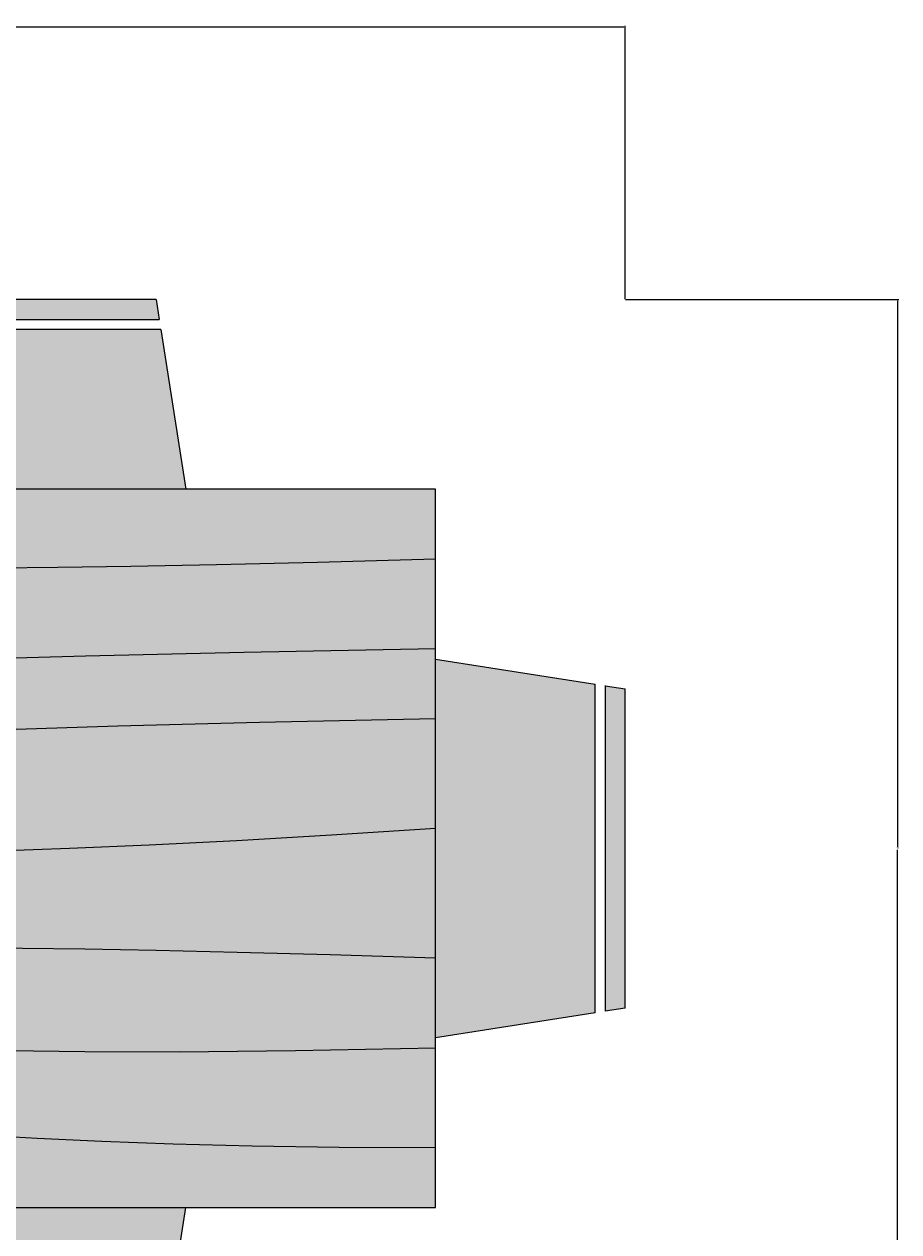
# Model space of a CAD drawing. Units: inches. Extents: x 192 to 1361, y -1362 to 367.
# Tile 18 of 23: x 662 to 781, y -337 to -173. Entities that reach past the tile are written whole.
import ezdxf

# ---------------------------------------------------------------- set-up
doc = ezdxf.new("R2010")
doc.units = ezdxf.units.IN
doc.header["$MEASUREMENT"] = 0
doc.layers.add('A-ANNO-DIMS', color=2, linetype='Continuous', lineweight=18)
doc.layers.add('furniture', color=32, linetype='Continuous', lineweight=18)
doc.layers.add('A-FURN-PATT', color=254, linetype='Continuous', lineweight=13, true_color=0xfeeab9)
doc.styles.get("Standard").update_dxf_attribs({"font": 'arial.ttf'})
doc.dimstyles.get("Standard").update_dxf_attribs({"dimtxt": 0.18, "dimasz": 0.18, "dimexe": 0.18, "dimexo": 0.0625, "dimgap": 0.09, "dimtad": 0, "dimtih": 1, "dimtoh": 1, "dimzin": 0, "dimdsep": 46, "dimlunit": 3, "dimtxsty": 'Standard', "dimcen": 0.09, "dimadec": 0, "dimazin": 0, "dimtfac": 1, "dimtofl": 0, "dimtmove": 0, "dimatfit": 3, "dimfxl": 1, "dimtolj": 1, "dimtzin": 0, "dimarcsym": 0})

# ---------------------------------------------------------------- blocks, each defined once
blk = doc.blocks.new('Dining Set - 36 x 72 in.')
for p, q in [((-22, 27.5), (-22.1562, 26.50042)), ((-22, 27.5), (-6, 27.5)), ((-5.8437, 26.49966), (-6, 27.5)), ((6, 27.5), (5.8438, 26.50042)), ((6, 27.5), (22, 27.5)), ((22.1563, 26.49966), (22, 27.5)), ((-5.8416, 26.5), (-22.1534, 26.5)), ((22.1584, 26.5), (5.8466, 26.5)), ((-22.2343, 26.00059), (-23.4847, 17.99762)), ((-22.2304, 26), (-5.7608, 26)), ((-4.5152, 17.99762), (-5.7655, 25.99926)), ((5.7657, 26.00059), (4.5153, 17.99762)), ((5.7696, 26), (22.2392, 26)), ((23.4848, 17.99762), (22.2345, 25.99926)), ((36, 18), (-36, 18)), ((-36, 18), (-36, -18)), ((36, -18), (36, 18)), ((-44.0006, 8.23428), (-35.9976, 9.48474)), ((44.0006, 8.23428), (35.9976, 9.48474)), ((-45.5, 8), (-44.5004, 8.15617)), ((-45.5, 8), (-45.5, -8)), ((-44.5, -8.15843), (-44.5, 8.15338)), ((-44, 8.23041), (-44, -8.23915)), ((44, 8.23041), (44, -8.23915)), ((44.5, -8.15843), (44.5, 8.15338)), ((45.5, 8), (44.5005, 8.15617)), ((45.5, 8), (45.5, -8)), ((-44.4997, -8.15631), (-45.5, -8)), ((-35.9976, -9.48476), (-43.9993, -8.2345)), ((35.9976, -9.48476), (43.9993, -8.2345)), ((44.4997, -8.15631), (45.5, -8)), ((-36, -18), (36, -18)), ((-22.2343, -26.0006), (-23.4847, -17.99762)), ((-4.5152, -17.99762), (-5.7655, -25.99928)), ((5.7657, -26.0006), (4.5153, -17.99762)), ((23.4848, -17.99762), (22.2345, -25.99928)), ((-22.2304, -26), (-5.7608, -26)), ((5.7696, -26), (22.2392, -26)), ((-22, -27.5), (-22.1562, -26.50044)), ((-5.8416, -26.5), (-22.1534, -26.5)), ((-5.8437, -26.49967), (-6, -27.5)), ((6, -27.5), (5.8438, -26.50044)), ((22.1584, -26.5), (5.8466, -26.5)), ((22.1563, -26.49967), (22, -27.5)), ((-22, -27.5), (-6, -27.5)), ((6, -27.5), (22, -27.5))]:
    blk.add_line(p, q)
for points in [[(-36, 15), (-31.1772, 14.97754), (-26.8079, 14.91406), (-22.8538, 14.81543), (-19.276, 14.6875), (-16.0362, 14.53613), (-13.0957, 14.36718), (-10.4159, 14.18652), (-7.9583, 14), (-5.6904, 13.81315), (-3.6035, 13.63021), (-1.6954, 13.45508), (0.0365, 13.29166), (1.5945, 13.14388), (2.9811, 13.01562), (4.1988, 12.9108), (5.25, 12.83333), (6.1393, 12.78613), (6.8802, 12.76823), (7.4883, 12.77767), (7.9792, 12.8125), (8.3685, 12.87077), (8.6719, 12.95052), (8.9049, 13.0498), (9.0833, 13.16666), (9.2205, 13.29899), (9.3216, 13.44401), (9.3895, 13.59879), (9.4271, 13.76041), (9.4373, 13.92594), (9.4232, 14.09245), (9.3875, 14.257), (9.3333, 14.41666), (9.2638, 14.56917), (9.1836, 14.71484), (9.0975, 14.85465), (9.0104, 14.98958), (8.9272, 15.1206), (8.8529, 15.2487), (8.7922, 15.37483), (8.75, 15.5), (8.7305, 15.62467), (8.7344, 15.74739), (8.7617, 15.86621), (8.8125, 15.97916), (8.8867, 16.08431), (8.9844, 16.17968), (9.1055, 16.26334), (9.25, 16.33333), (9.4189, 16.38802), (9.6172, 16.42708), (9.8506, 16.45052), (10.125, 16.45833), (10.4463, 16.45052), (10.8203, 16.42708), (11.2529, 16.38802), (11.75, 16.33333), (12.3184, 16.26318), (12.9694, 16.17838), (13.7151, 16.07991), (14.5677, 15.96875), (15.5395, 15.84586), (16.6426, 15.71224), (17.8893, 15.56884), (19.2917, 15.41666), (20.859, 15.25667), (22.5879, 15.08984), (24.4721, 14.91715), (26.5052, 14.73958), (28.6809, 14.5581), (30.9929, 14.3737), (33.4347, 14.18733), (36, 14)], [(-36, 10), (-28.9766, 10.14274), (-23.1725, 10.20442), (-18.4241, 10.19775), (-14.5677, 10.13541), (-11.4399, 10.03011), (-8.877, 9.89453), (-6.7154, 9.74137), (-4.7917, 9.58333), (-2.9698, 9.43082), (-1.2246, 9.28515), (0.4415, 9.14534), (2.026, 9.01041), (3.5266, 8.87939), (4.9408, 8.7513), (6.266, 8.62516), (7.5, 8.5), (8.6411, 8.37549), (9.6914, 8.2539), (10.6538, 8.13818), (11.5312, 8.03125), (12.3267, 7.93603), (13.043, 7.85547), (13.6831, 7.79248), (14.25, 7.75), (14.7471, 7.7303), (15.1797, 7.73307), (15.5537, 7.75732), (15.875, 7.80208), (16.1494, 7.86637), (16.3828, 7.94922), (16.5811, 8.04964), (16.75, 8.16666), (16.8944, 8.29915), (17.0143, 8.44531), (17.1089, 8.60319), (17.1771, 8.77083), (17.218, 8.94629), (17.2305, 9.1276), (17.2137, 9.31282), (17.1667, 9.5), (17.0895, 9.6875), (16.987, 9.875), (16.8649, 10.0625), (16.7292, 10.25), (16.5856, 10.4375), (16.4401, 10.625), (16.2985, 10.8125), (16.1667, 11), (16.05, 11.18733), (15.9518, 11.3737), (15.8752, 11.5581), (15.8229, 11.73958), (15.798, 11.91715), (15.8034, 12.08984), (15.842, 12.25667), (15.9167, 12.41666), (16.0295, 12.56836), (16.1784, 12.70833), (16.3605, 12.83268), (16.5729, 12.9375), (16.8127, 13.01888), (17.0768, 13.07291), (17.3625, 13.0957), (17.6667, 13.08333), (17.9894, 13.03312), (18.3418, 12.94726), (18.7382, 12.82918), (19.1927, 12.68229), (19.7195, 12.51001), (20.3327, 12.31575), (21.0465, 12.10294), (21.875, 11.875), (22.8357, 11.63354), (23.959, 11.37304), (25.2786, 11.08618), (26.8282, 10.76562), (28.6414, 10.40405), (30.752, 9.99414), (33.1936, 9.52856), (36, 9)], [(-36, 5.5), (-30.7157, 5.3348), (-26.069, 5.20963), (-21.9946, 5.11767), (-18.4271, 5.05208), (-15.3009, 5.00602), (-12.5508, 4.97265), (-10.1112, 4.94515), (-7.9167, 4.91666), (-5.909, 4.88167), (-4.0586, 4.83984), (-2.3429, 4.79215), (-0.7396, 4.73958), (0.7739, 4.6831), (2.22, 4.6237), (3.6213, 4.56233), (5, 4.5), (6.373, 4.43782), (7.7344, 4.3776), (9.0723, 4.32129), (10.375, 4.27083), (11.6309, 4.22819), (12.8281, 4.19531), (13.9551, 4.17415), (15, 4.16666), (15.954, 4.17448), (16.819, 4.19791), (17.6001, 4.23698), (18.3021, 4.29166), (18.9299, 4.36198), (19.4883, 4.44791), (19.9823, 4.54948), (20.4167, 4.66666), (20.7969, 4.79899), (21.1302, 4.94401), (21.4245, 5.09879), (21.6875, 5.26041), (21.9271, 5.42594), (22.1511, 5.59245), (22.3672, 5.757), (22.5834, 5.91666), (22.8065, 6.06868), (23.0404, 6.21093), (23.2879, 6.34147), (23.5521, 6.45833), (23.8358, 6.55957), (24.142, 6.64323), (24.4735, 6.70735), (24.8334, 6.75), (25.2235, 6.76969), (25.642, 6.76692), (26.0858, 6.74267), (26.5521, 6.69791), (27.0379, 6.63362), (27.5404, 6.55078), (28.0565, 6.45036), (28.5834, 6.33333), (29.1242, 6.19987), (29.7071, 6.04687), (30.3661, 5.87044), (31.1354, 5.66666), (32.0493, 5.43164), (33.142, 5.16146), (34.4475, 4.85221), (36, 4.5)], [(-36, -1), (-30.7915, -0.6591), (-26.0195, -0.38216), (-21.6519, -0.16284), (-17.6563, 0.00521), (-14.0005, 0.12833), (-10.6523, 0.21289), (-7.5796, 0.26522), (-4.75, 0.29166), (-2.134, 0.29793), (0.2878, 0.28711), (2.5317, 0.26163), (4.6146, 0.22396), (6.5529, 0.17651), (8.3633, 0.12174), (10.0623, 0.06209), (11.6667, 0), (13.1899, -0.06201), (14.6341, -0.1211), (15.9982, -0.17432), (17.2813, -0.21875), (18.4823, -0.25147), (19.6003, -0.26953), (20.6343, -0.27002), (21.5834, -0.25), (22.4481, -0.20768), (23.2357, -0.14584), (23.9549, -0.06836), (24.6146, 0.02083), (25.2235, 0.11784), (25.7904, 0.21875), (26.3241, 0.31966), (26.8334, 0.41666), (27.3265, 0.50618), (27.8099, 0.58593), (28.2894, 0.65397), (28.7709, 0.70833), (29.2601, 0.74707), (29.763, 0.76823), (30.2855, 0.76985), (30.8334, 0.75), (31.4088, 0.70784), (31.9994, 0.64713), (32.589, 0.57275), (33.1615, 0.48958), (33.7008, 0.4025), (34.1908, 0.3164), (34.6153, 0.23616), (34.9584, 0.16666), (35.2099, 0.11165), (35.3848, 0.07031), (35.504, 0.04069), (35.5886, 0.02083), (35.6594, 0.00879), (35.7377, 0.0026), (35.8442, 0.00032), (36, 0)], [(-36, -6.5), (-27.1843, -6.31267), (-20.084, -6.1263), (-14.469, -5.9419), (-10.1094, -5.76042), (-6.7752, -5.58285), (-4.2363, -5.41016), (-2.2629, -5.24333), (-0.625, -5.08334), (0.8708, -4.93099), (2.2715, -4.78646), (3.5872, -4.64974), (4.8281, -4.52084), (6.0046, -4.39974), (7.127, -4.28646), (8.2053, -4.18099), (9.25, -4.08334), (10.2705, -3.99382), (11.2734, -3.91407), (12.2647, -3.84603), (13.25, -3.79167), (14.2354, -3.75293), (15.2266, -3.73177), (16.2295, -3.73015), (17.25, -3.75), (18.2912, -3.79248), (19.3451, -3.85547), (20.4009, -3.93604), (21.4479, -4.03125), (22.4754, -4.13819), (23.4727, -4.25391), (24.4289, -4.37549), (25.3334, -4.5), (26.1785, -4.62492), (26.9694, -4.74935), (27.7145, -4.87281), (28.4219, -4.99479), (29.1, -5.11483), (29.7572, -5.23242), (30.4016, -5.34709), (31.0417, -5.45834), (31.6837, -5.56437), (32.3262, -5.65821), (32.9658, -5.73153), (33.599, -5.77604), (34.2224, -5.78345), (34.8327, -5.74545), (35.4264, -5.65373), (36, -5.5)], [(-36, -10), (-26.4022, -9.81299), (-18.4675, -9.62891), (-11.9839, -9.45069), (-6.7396, -9.28125), (-2.5226, -9.12354), (0.8789, -8.98047), (3.6769, -8.85498), (6.0833, -8.75), (8.2767, -8.66765), (10.3021, -8.60677), (12.1712, -8.56543), (13.8958, -8.54167), (15.4876, -8.53353), (16.9583, -8.53907), (18.3197, -8.55632), (19.5834, -8.58334), (20.7616, -8.61841), (21.8685, -8.66081), (22.9188, -8.71004), (23.9271, -8.76563), (24.9081, -8.82707), (25.8763, -8.89388), (26.8465, -8.96558), (27.8334, -9.04167), (28.8474, -9.12118), (29.8828, -9.20117), (30.93, -9.27824), (31.9792, -9.34896), (33.0205, -9.40991), (34.0443, -9.45768), (35.0407, -9.48885), (36, -9.5)], [(-36, -14.5), (-30.0881, -14.33513), (-25.0332, -14.21224), (-20.7312, -14.12647), (-17.0781, -14.07292), (-13.97, -14.04671), (-11.3027, -14.04297), (-8.9724, -14.05681), (-6.875, -14.08334), (-4.9224, -14.11833), (-3.0905, -14.16016), (-1.3709, -14.20785), (0.2448, -14.26042), (1.7647, -14.3169), (3.1973, -14.3763), (4.5507, -14.43767), (5.8333, -14.5), (7.0554, -14.5621), (8.235, -14.62175), (9.3922, -14.67652), (10.5469, -14.72396), (11.7192, -14.76164), (12.929, -14.78711), (14.1965, -14.79794), (15.5417, -14.79167), (16.9933, -14.76424), (18.6152, -14.70508), (20.4804, -14.60197), (22.6615, -14.44271), (25.2312, -14.21509), (28.2624, -13.9069), (31.8277, -13.50594), (36, -13)]]:
    blk.add_lwpolyline(points)
blk = doc.blocks.new('dining area')
at = {"layer": 'furniture', "xscale": 0.6659924291999282, "yscale": 0.6659924291999282, "zscale": 0.6659924291999282, "rotation": 90}
blk.add_blockref('Dining Set - 36 x 72 in.', (-0.439, 20.507), dxfattribs=at)
blk = doc.blocks.new('*D43')
at = {"layer": 'A-ANNO-DIMS', "color": 0, "lineweight": -2, "transparency": 16777216}
for p, q in [((497.85, -210.68), (497.85, -173.69)), ((498.03, -173.87), (619.71, -173.87)), ((743.46, -173.87), (621.79, -173.87)), ((743.64, -210.68), (743.64, -173.69))]:
    blk.add_line(p, q, dxfattribs=at)
at = {"layer": 'A-ANNO-DIMS', "color": 0, "transparency": 16777216}
for points in [[(498.03, -173.84), (498.03, -173.9), (497.85, -173.87)], [(743.46, -173.84), (743.46, -173.9), (743.64, -173.87)]]:
    blk.add_solid(points, dxfattribs=at)
at = {"layer": 'Defpoints', "color": 0, "transparency": 16777216}
for p in [(497.85, -173.87), (497.85, -210.74), (743.64, -210.74)]:
    blk.add_point(p, dxfattribs=at)
at = {"layer": 'A-ANNO-DIMS', "color": 0, "transparency": 16777216, "insert": (620.75, -173.87), "char_height": 0.18, "attachment_point": 5}
blk.add_mtext('\\A1;DINING SET 246', dxfattribs=at)
blk = doc.blocks.new('*D44')
at = {"layer": 'A-ANNO-DIMS', "color": 0, "lineweight": -2, "transparency": 16777216}
for p, q in [((743.7, -210.74), (780.69, -210.74)), ((780.51, -210.92), (780.51, -284.83)), ((780.51, -359.11), (780.51, -285.2)), ((743.7, -359.29), (780.69, -359.29))]:
    blk.add_line(p, q, dxfattribs=at)
at = {"layer": 'A-ANNO-DIMS', "color": 0, "transparency": 16777216}
for points in [[(780.48, -210.92), (780.54, -210.92), (780.51, -210.74)], [(780.48, -359.11), (780.54, -359.11), (780.51, -359.29)]]:
    blk.add_solid(points, dxfattribs=at)
at = {"layer": 'Defpoints', "color": 0, "transparency": 16777216}
for p in [(743.64, -210.74), (780.51, -210.74), (743.64, -359.29)]:
    blk.add_point(p, dxfattribs=at)
at = {"layer": 'A-ANNO-DIMS', "color": 0, "transparency": 16777216, "insert": (780.51, -285.01), "char_height": 0.18, "attachment_point": 5}
blk.add_mtext('\\A1;149', dxfattribs=at)

msp = doc.modelspace()

# ---------------------------------------------------------------- hatches: boundary and pattern name
at = {"layer": 'A-FURN-PATT'}
h = msp.add_hatch(color=256, dxfattribs=at)
h.dxf.hatch_style = 1
h.paths.add_polyline_path([(605.1742, -214.7906), (560.6934, -214.7906), (557.3171, -236.398), (608.5502, -236.398)])
h.paths.add_polyline_path([(604.5412, -210.7392), (561.3264, -210.7392), (560.9044, -213.4402), (604.9632, -213.4402)])
h.paths.add_polyline_path([(680.8, -214.7906), (636.3191, -214.7906), (632.9429, -236.398), (684.176, -236.398)])
h.paths.add_polyline_path([(680.1669, -210.7392), (636.9522, -210.7392), (636.5302, -213.4402), (680.589, -213.4402)])
h.paths.add_polyline_path([(523.5135, -259.398), (501.9062, -262.7741), (501.9062, -307.2549), (523.5135, -310.6311)])
h.paths.add_polyline_path([(500.5557, -262.9851), (497.8548, -263.4072), (497.8548, -306.6219), (500.5557, -307.0439)])
h.paths.add_polyline_path([(608.5502, -333.6311), (557.3171, -333.6311), (560.6934, -355.2385), (605.1742, -355.2385)])
h.paths.add_polyline_path([(604.9632, -356.5889), (560.9044, -356.5889), (561.3264, -359.2899), (604.5412, -359.2899)])
h.paths.add_polyline_path([(680.589, -356.5889), (636.5302, -356.5889), (636.9522, -359.2899), (680.1669, -359.2899)])
h.paths.add_polyline_path([(684.176, -333.6311), (632.9429, -333.6311), (636.3191, -355.2385), (680.8, -355.2385)])
h.paths.add_polyline_path([(739.5872, -262.7741), (717.9798, -259.398), (717.9798, -310.6311), (739.5872, -307.2549)])
h.paths.add_polyline_path([(743.6386, -263.4072), (740.9376, -262.9851), (740.9376, -307.0439), (743.6386, -306.6219)])
h = msp.add_hatch(color=256, dxfattribs=at)
h.dxf.hatch_style = 1
h.paths.add_polyline_path([(717.9798, -236.398), (523.5135, -236.398), (523.5135, -249.9026), (534.7826, -248.5361), (544.4122, -247.4531), (552.5992, -246.6207), (559.5398, -246.0059), (565.4307, -245.5758), (570.4685, -245.2973), (574.8491, -245.1375), (578.7698, -245.0634), (582.4031, -245.0465), (585.8265, -245.0757), (589.094, -245.1445), (592.2603, -245.2463), (595.3791, -245.3744), (598.5046, -245.5224), (601.6906, -245.6835), (604.9914, -245.8512), (608.4556, -246.0195), (612.111, -246.1853), (615.9804, -246.3457), (620.0855, -246.4983), (624.4494, -246.6403), (629.0939, -246.7691), (634.0417, -246.8821), (639.3155, -246.9766), (644.9804, -247.0482), (651.2744, -247.0856), (658.4785, -247.0755), (666.8733, -247.0047), (676.74, -246.8601), (688.3594, -246.6284), (702.0122, -246.2965), (717.9798, -245.8512)])
h.paths.add_polyline_path([(717.9798, -245.8512), (702.0122, -246.2965), (688.3594, -246.6284), (676.74, -246.8601), (666.8733, -247.0047), (658.4785, -247.0755), (651.2744, -247.0856), (644.9804, -247.0482), (639.3155, -246.9766), (634.0417, -246.8821), (629.0939, -246.7691), (624.4494, -246.6403), (620.0855, -246.4983), (615.9804, -246.3457), (612.111, -246.1853), (608.4556, -246.0195), (604.9914, -245.8512), (601.6906, -245.6835), (598.5046, -245.5224), (595.3791, -245.3744), (592.2603, -245.2463), (589.094, -245.1445), (585.8265, -245.0757), (582.4031, -245.0465), (578.7698, -245.0634), (574.8491, -245.1375), (570.4685, -245.2973), (565.4307, -245.5758), (559.5398, -246.0059), (552.5992, -246.6207), (544.4122, -247.4531), (534.7826, -248.5361), (523.5135, -249.9026), (523.5135, -259.3558), (526.1045, -259.3859), (528.7957, -259.4701), (531.5609, -259.5991), (534.3734, -259.7638), (537.2072, -259.9548), (540.0356, -260.1629), (542.8321, -260.379), (545.5709, -260.5937), (548.2364, -260.7992), (550.8568, -260.9929), (553.4719, -261.1733), (556.1215, -261.3393), (558.8448, -261.4894), (561.6816, -261.6224), (564.6712, -261.7369), (567.8535, -261.8316), (571.2666, -261.9046), (574.9437, -261.9512), (578.9159, -261.9662), (583.2152, -261.9442), (587.8732, -261.88), (592.9215, -261.7683), (598.392, -261.6039), (604.3162, -261.3815), (610.8157, -261.098), (618.3728, -260.759), (627.56, -260.3726), (638.9498, -259.9466), (653.1142, -259.489), (670.6259, -259.0076), (692.0569, -258.5104), (717.9798, -258.0053)])
h.paths.add_polyline_path([(602.4999, -265.0738), (602.0375, -261.467), (598.392, -261.6039), (592.9215, -261.7683), (587.8732, -261.88), (583.2152, -261.9442), (578.9159, -261.9662), (574.9437, -261.9512), (571.2666, -261.9046), (567.8535, -261.8316), (564.6712, -261.7369), (561.6816, -261.6224), (558.8448, -261.4894), (556.1215, -261.3393), (553.4719, -261.1733), (550.8568, -260.9929), (548.2364, -260.7992), (545.5709, -260.5937), (542.8321, -260.379), (540.0356, -260.1629), (537.2072, -259.9548), (534.3734, -259.7638), (531.5609, -259.5991), (528.7957, -259.4701), (526.1045, -259.3859), (523.7648, -259.3587), (523.5135, -259.398), (523.5135, -270.1595), (525.0628, -269.7443), (526.6663, -269.4965), (528.3147, -269.3939), (529.9984, -269.4139), (531.7087, -269.5341), (533.4362, -269.7322), (535.1715, -269.9856), (536.9055, -270.272), (538.6344, -270.5725), (540.3748, -270.8822), (542.1499, -271.1998), (543.9814, -271.524), (545.892, -271.8535), (547.9045, -272.1869), (550.0406, -272.523), (552.3232, -272.8604), (554.7662, -273.1967), (557.3488, -273.5251), (560.0424, -273.8376), (562.8176, -274.1265), (565.6455, -274.3836), (568.4971, -274.6012), (571.3436, -274.7714), (574.1558, -274.8861), (576.9121, -274.9397), (579.6208, -274.9353), (582.298, -274.8782), (584.9595, -274.7735), (587.6207, -274.6267), (590.2981, -274.443), (593.0069, -274.2276), (595.7632, -273.9858), (598.5848, -273.722), (601.4972, -273.4372), (604.5287, -273.1312), (607.7064, -272.8041), (611.0579, -272.456), (611.8813, -272.3704)])
h.paths.add_polyline_path([(613.2364, -275.1581), (604.0875, -273.1757), (601.4972, -273.4372), (598.5848, -273.722), (595.7632, -273.9858), (593.0069, -274.2276), (590.2981, -274.443), (587.6207, -274.6267), (584.9595, -274.7735), (582.298, -274.8782), (579.6208, -274.9353), (576.9121, -274.9397), (574.1558, -274.8861), (571.3436, -274.7714), (568.4971, -274.6012), (565.6455, -274.3836), (562.8176, -274.1265), (560.0424, -273.8376), (557.3488, -273.5251), (554.7662, -273.1967), (552.3232, -272.8604), (550.0406, -272.523), (547.9045, -272.1869), (545.892, -271.8535), (543.9814, -271.524), (542.1499, -271.1998), (540.3748, -270.8822), (538.6344, -270.5725), (536.9055, -270.272), (535.1715, -269.9856), (533.4362, -269.7322), (531.7087, -269.5341), (529.9984, -269.4139), (528.3147, -269.3939), (526.6663, -269.4965), (525.0628, -269.7443), (523.5135, -270.1595), (523.5135, -285.0145), (524.3927, -285.0164), (524.8532, -285.1244), (525.1751, -285.2045), (525.6475, -285.3161), (526.3268, -285.4647), (527.2535, -285.6524), (528.4, -285.8691), (529.7235, -286.1017), (531.1801, -286.3369), (532.7264, -286.5615), (534.3188, -286.7624), (535.914, -286.9264), (537.4681, -287.0402), (538.9479, -287.0939), (540.3592, -287.0895), (541.7175, -287.0323), (543.0388, -286.9277), (544.3393, -286.7809), (545.6343, -286.5971), (546.94, -286.3817), (548.2718, -286.1399), (549.6474, -285.8779), (551.0889, -285.6054), (552.62, -285.3328), (554.2646, -285.0708), (556.0464, -284.8299), (557.9889, -284.6206), (560.1161, -284.4536), (562.4516, -284.3393), (565.0151, -284.2852), (567.8078, -284.2866), (570.8275, -284.3353), (574.0713, -284.4237), (577.5368, -284.5437), (581.2211, -284.6875), (585.1218, -284.8471), (589.2358, -285.0145), (593.5692, -285.1822), (598.1581, -285.3434), (603.0478, -285.4913), (608.283, -285.6194), (613.9088, -285.7212), (616.4226, -285.7497), (616.7471, -285.69)], flags=16)
h.paths.add_polyline_path([(717.9798, -258.0053), (692.0569, -258.5104), (670.6259, -259.0076), (653.1142, -259.489), (638.9498, -259.9466), (627.56, -260.3726), (618.3728, -260.759), (610.8157, -261.098), (604.3162, -261.3815), (602.0375, -261.467), (602.4999, -265.0738), (611.8813, -272.3704), (614.6115, -272.0867), (618.3947, -271.6963), (622.4348, -271.2849), (627.3208, -270.8076), (627.3197, -270.8137), (632.1886, -270.4021), (639.046, -269.9357), (648.0514, -269.4561), (659.8263, -268.9659), (674.992, -268.4679), (694.1693, -267.9645), (717.9798, -267.4586)])
h.paths.add_polyline_path([(717.9798, -267.4586), (694.1693, -267.9645), (674.992, -268.4679), (659.8263, -268.9659), (648.0514, -269.4561), (639.046, -269.9357), (637.7073, -270.0268), (634.981, -274.8872), (634.93, -274.8716), (627.474, -277.1084), (618.2223, -284.5098), (623.8182, -285.8072), (626.5104, -285.8192), (633.576, -285.8023), (641.2186, -285.7309), (649.5177, -285.5895), (658.5609, -285.3612), (668.4349, -285.0286), (679.2267, -284.5747), (691.0233, -283.9824), (703.9121, -283.2344), (717.9798, -282.3136)])
h.paths.add_polyline_path([(717.9798, -282.3136), (703.9121, -283.2344), (691.0233, -283.9824), (679.2267, -284.5747), (668.4349, -285.0286), (658.5609, -285.3612), (649.5177, -285.5895), (641.2186, -285.7309), (633.576, -285.8023), (626.5104, -285.8192), (619.9694, -285.79), (616.8026, -285.7541), (623.8185, -293.8493), (623.9185, -293.8319), (623.9419, -293.9917), (626.0437, -296.4169), (628.742, -298.0041), (631.7086, -298.0866), (636.7064, -298.1996), (642.1291, -298.2941), (648.0562, -298.371), (654.6454, -298.4453), (662.0732, -298.5354), (670.5168, -298.6598), (680.1523, -298.837), (691.157, -299.0853), (703.7073, -299.4234), (717.9798, -299.8696)])
h.paths.add_polyline_path([(717.9798, -299.8696), (703.7073, -299.4234), (691.157, -299.0853), (680.1523, -298.837), (670.5168, -298.6598), (662.0732, -298.5354), (654.6454, -298.4453), (648.0562, -298.371), (642.1291, -298.2941), (636.7064, -298.1996), (631.7086, -298.0866), (628.742, -298.0041), (626.0437, -296.4169), (623.9419, -293.9917), (616.8026, -285.7541), (616.738, -285.7533), (614.6017, -300.7077), (613.756, -301.5533), (614.1357, -309.2515), (615.2746, -309.351), (619.5542, -309.7154), (624.0542, -310.093), (628.7679, -310.4864), (633.6887, -310.8984), (638.8844, -311.3252), (644.7227, -311.7389), (651.6449, -312.1051), (660.0929, -312.3895), (670.5087, -312.5579), (683.3338, -312.5759), (699.0102, -312.4093), (717.9798, -312.0238)], flags=17)
h.paths.add_polyline_path([(615.758, -292.6135), (616.7471, -285.69), (613.2364, -275.1581), (604.0875, -273.1757), (601.4972, -273.4372), (598.5848, -273.722), (595.7632, -273.9858), (593.0069, -274.2276), (590.2981, -274.443), (587.6207, -274.6267), (584.9595, -274.7735), (582.298, -274.8782), (579.6208, -274.9353), (576.9121, -274.9397), (574.1558, -274.8861), (571.3436, -274.7714), (568.4971, -274.6012), (565.6455, -274.3836), (562.8176, -274.1265), (560.0424, -273.8376), (557.3488, -273.5251), (554.7662, -273.1967), (552.3232, -272.8604), (550.0406, -272.523), (547.9045, -272.1869), (545.892, -271.8535), (543.9814, -271.524), (542.1499, -271.1998), (540.3748, -270.8822), (538.6344, -270.5725), (536.9055, -270.272), (535.1715, -269.9856), (533.4362, -269.7322), (531.7087, -269.5341), (529.9984, -269.4139), (528.3147, -269.3939), (526.6663, -269.4965), (525.0628, -269.7443), (523.5135, -270.1595), (523.5135, -285.0145), (524.3927, -285.0164), (524.8532, -285.1244), (525.1751, -285.2045), (525.9724, -285.3929), (526.3268, -285.4647), (525.4551, -285.274), (524.8532, -285.1244), (524.3927, -285.0164), (523.5135, -285.0145), (523.5135, -297.1687), (527.7067, -298.12), (531.2328, -298.9552), (534.1841, -299.685), (536.6524, -300.3197), (538.7303, -300.8701), (540.5102, -301.3467), (542.0845, -301.7599), (543.5452, -302.1204), (544.9683, -302.4365), (546.3622, -302.7077), (547.7195, -302.9314), (549.0316, -303.1051), (550.291, -303.226), (551.4897, -303.2915), (552.62, -303.2989), (553.6736, -303.2458), (554.6457, -303.1306), (555.5411, -302.9574), (556.3681, -302.7314), (557.1343, -302.458), (557.8479, -302.1424), (558.5164, -301.7898), (559.1481, -301.4056), (559.7507, -300.995), (560.3346, -300.5637), (561.3682, -299.7768), (562.1705, -299.2225), (562.8808, -298.786), (563.6757, -298.3679), (564.5759, -297.9762), (565.6028, -297.6188), (566.7761, -297.3023), (568.1103, -297.028), (569.6185, -296.7959), (571.3142, -296.606), (573.2102, -296.4583), (575.3199, -296.3528), (577.6562, -296.2895), (580.2329, -296.2684), (583.0551, -296.2886), (586.099, -296.3457), (589.3325, -296.4346), (592.7246, -296.5497), (596.2431, -296.686), (599.8567, -296.8381), (603.5337, -297.0007), (607.2421, -297.1687), (609.1466, -297.2548)])
h.paths.add_polyline_path([(614.6017, -300.7077), (615.758, -292.6135), (609.1466, -297.2548), (607.2421, -297.1687), (603.5337, -297.0007), (599.8567, -296.8381), (596.2431, -296.686), (592.7246, -296.5497), (589.3325, -296.4346), (586.099, -296.3457), (583.0551, -296.2886), (580.2329, -296.2684), (577.6562, -296.2895), (575.3199, -296.3528), (573.2102, -296.4583), (571.3142, -296.606), (569.6185, -296.7959), (568.1103, -297.028), (566.7761, -297.3023), (565.6028, -297.6188), (564.5759, -297.9762), (563.6757, -298.3679), (562.8808, -298.786), (562.1705, -299.2225), (561.3682, -299.7768), (559.9183, -300.8808), (558.8169, -301.6313), (557.8479, -302.1424), (557.1343, -302.458), (556.3681, -302.7314), (555.5411, -302.9574), (554.6457, -303.1306), (553.6736, -303.2458), (552.62, -303.2989), (551.4897, -303.2915), (550.291, -303.226), (549.0316, -303.1051), (547.7195, -302.9314), (546.3622, -302.7077), (544.9683, -302.4365), (543.5452, -302.1204), (542.0845, -301.7599), (540.5102, -301.3467), (538.7303, -300.8701), (536.6524, -300.3197), (534.1841, -299.685), (531.2328, -298.9552), (527.7067, -298.12), (523.5135, -297.1687), (523.5135, -309.3228), (531.0934, -310.7504), (537.688, -312.0079), (543.3885, -313.1151), (548.2858, -314.0916), (552.4712, -314.9574), (556.0353, -315.7322), (559.0693, -316.4358), (561.664, -317.088), (563.9018, -317.7036), (565.8297, -318.2784), (567.4859, -318.8031), (568.9087, -319.2684), (570.1363, -319.6651), (571.2069, -319.9841), (572.1587, -320.216), (573.0303, -320.3516), (573.8519, -320.385), (574.6236, -320.3234), (575.3369, -320.1775), (575.9846, -319.9577), (576.5583, -319.6746), (577.0501, -319.3387), (577.4523, -318.9607), (577.7569, -318.551), (577.9587, -318.1188), (578.0629, -317.6682), (578.0775, -317.2018), (578.0103, -316.7222), (577.869, -316.2321), (577.6621, -315.734), (577.3969, -315.2306), (577.0817, -314.7247), (576.7257, -314.2183), (576.3433, -313.7118), (575.6335, -312.7972), (574.9795, -311.8936), (574.4388, -310.9045), (574.1912, -309.9182), (574.259, -308.9341), (574.6297, -308.023), (575.2828, -307.2269), (576.2025, -306.5897), (577.1284, -306.261), (577.8696, -306.0873), (578.7374, -305.9665), (579.7475, -305.901), (580.9159, -305.8935), (582.2586, -305.9467), (583.7897, -306.0614), (585.5186, -306.2315), (587.4532, -306.4491), (589.6018, -306.7063), (591.9716, -306.9951), (594.571, -307.3077), (597.4078, -307.6361), (600.4898, -307.9724), (603.8227, -308.3104), (606.7229, -308.5865)], flags=0)
h.paths.add_polyline_path([(613.2364, -275.1581), (604.0875, -273.1757), (601.4972, -273.4372), (598.5848, -273.722), (595.7632, -273.9858), (593.0069, -274.2276), (590.2981, -274.443), (587.6207, -274.6267), (584.9595, -274.7735), (582.298, -274.8782), (579.6208, -274.9353), (576.9121, -274.9397), (574.1558, -274.8861), (571.3436, -274.7714), (568.4971, -274.6012), (565.6455, -274.3836), (562.8176, -274.1265), (560.0424, -273.8376), (557.3488, -273.5251), (554.7662, -273.1967), (552.3232, -272.8604), (550.0406, -272.523), (547.9045, -272.1869), (545.892, -271.8535), (543.9814, -271.524), (542.1499, -271.1998), (540.3748, -270.8822), (538.6344, -270.5725), (536.9055, -270.272), (535.1715, -269.9856), (533.4362, -269.7322), (531.7087, -269.5341), (529.9984, -269.4139), (528.3147, -269.3939), (526.6663, -269.4965), (525.0628, -269.7443), (523.5135, -270.1595), (523.5135, -285.0145), (523.9343, -285.0154), (524.3927, -285.0164), (524.8532, -285.1244), (525.1751, -285.2045), (525.6475, -285.3161), (526.3268, -285.4647), (527.2535, -285.6524), (528.4, -285.8691), (529.7235, -286.1017), (531.1801, -286.3369), (532.7264, -286.5615), (534.3188, -286.7624), (535.914, -286.9264), (537.4681, -287.0402), (538.9479, -287.0939), (540.3592, -287.0895), (541.7175, -287.0323), (543.0388, -286.9277), (544.3393, -286.7809), (545.6343, -286.5971), (546.94, -286.3817), (548.2718, -286.1399), (549.6474, -285.8779), (551.0889, -285.6054), (552.62, -285.3328), (554.2646, -285.0708), (556.0464, -284.8299), (557.9889, -284.6206), (560.1161, -284.4536), (562.4516, -284.3393), (565.0151, -284.2852), (567.8078, -284.2866), (570.8275, -284.3353), (574.0713, -284.4237), (577.5368, -284.5437), (581.2211, -284.6875), (585.1218, -284.8471), (589.2358, -285.0145), (593.5692, -285.1822), (598.1581, -285.3434), (603.0478, -285.4913), (608.283, -285.6194), (613.9088, -285.7212), (616.4226, -285.7497), (616.7471, -285.69)], flags=17)
h.paths.add_polyline_path([(575.9846, -319.9577), (576.5583, -319.6746), (577.0501, -319.3387), (577.4523, -318.9607), (577.7569, -318.551), (577.9587, -318.1188), (578.0629, -317.6682), (578.0775, -317.2018), (578.0103, -316.7222), (577.869, -316.2321), (577.6621, -315.734), (577.3969, -315.2306), (577.0817, -314.7247), (576.7257, -314.2183), (576.3433, -313.7118), (575.3608, -312.4458), (575.1959, -312.1926), (574.9795, -311.8936), (574.4388, -310.9045), (574.1912, -309.9182), (574.259, -308.9341), (574.6297, -308.023), (575.2828, -307.2269), (576.2025, -306.5897), (577.1284, -306.261), (577.8696, -306.0873), (578.7374, -305.9665), (579.7475, -305.901), (580.9159, -305.8935), (582.2586, -305.9467), (583.7897, -306.0614), (585.5186, -306.2315), (587.4532, -306.4491), (589.6018, -306.7063), (591.9716, -306.9951), (594.571, -307.3077), (597.4078, -307.6361), (600.4898, -307.9724), (603.8227, -308.3104), (606.7229, -308.5865), (614.6017, -300.7077), (615.758, -292.6135), (609.1466, -297.2548), (607.2421, -297.1687), (603.5337, -297.0007), (599.8567, -296.8381), (596.2431, -296.686), (592.7246, -296.5497), (589.3325, -296.4346), (586.099, -296.3457), (583.0551, -296.2886), (580.2329, -296.2684), (577.6562, -296.2895), (575.3199, -296.3528), (573.2102, -296.4583), (571.3142, -296.606), (569.6185, -296.7959), (568.1103, -297.028), (566.7761, -297.3023), (565.6028, -297.6188), (564.5759, -297.9762), (563.6757, -298.3679), (562.8808, -298.786), (562.1705, -299.2225), (561.3682, -299.7768), (559.9183, -300.8808), (558.8169, -301.6313), (557.8479, -302.1424), (557.1343, -302.458), (556.3681, -302.7314), (555.5411, -302.9574), (554.6457, -303.1306), (553.6736, -303.2458), (552.62, -303.2989), (551.4897, -303.2915), (550.291, -303.226), (549.0316, -303.1051), (547.7195, -302.9314), (546.3622, -302.7077), (544.9683, -302.4365), (543.5452, -302.1204), (542.0845, -301.7599), (540.5102, -301.3467), (538.7303, -300.8701), (536.6524, -300.3197), (534.1841, -299.685), (531.2328, -298.9552), (527.7067, -298.12), (523.5135, -297.1687), (523.5135, -309.3228), (531.0934, -310.7504), (537.688, -312.0079), (543.3885, -313.1151), (548.2858, -314.0916), (552.4712, -314.9574), (556.0353, -315.7322), (559.0693, -316.4358), (561.664, -317.088), (563.9018, -317.7036), (565.8297, -318.2784), (567.4859, -318.8031), (568.9087, -319.2684), (570.1363, -319.6651), (571.2069, -319.9841), (572.1587, -320.216), (573.0303, -320.3516), (573.8519, -320.385), (574.6236, -320.3234), (575.3369, -320.1775)], flags=17)
h.paths.add_polyline_path([(606.7229, -308.5865), (603.8227, -308.3104), (600.4898, -307.9724), (597.4078, -307.6361), (594.571, -307.3077), (591.9716, -306.9951), (589.6018, -306.7063), (587.4532, -306.4491), (585.5186, -306.2315), (583.7897, -306.0614), (582.2586, -305.9467), (580.9159, -305.8935), (579.7475, -305.901), (578.7374, -305.9665), (577.8696, -306.0873), (577.1284, -306.261), (576.498, -306.4848), (575.9624, -306.756), (575.5063, -307.072), (575.1162, -307.4299), (574.7924, -307.8247), (574.5369, -308.2511), (574.3527, -308.7039), (574.2422, -309.1778), (574.2085, -309.6675), (574.2538, -310.1677), (574.3808, -310.6733), (574.5893, -311.1797), (574.8661, -311.6861), (575.1959, -312.1926), (575.5624, -312.699), (575.9503, -313.2054), (576.6244, -314.0741), (577.2758, -315.0008), (577.802, -315.9994), (578.0845, -316.9797), (578.0553, -317.9119), (577.6543, -318.7708), (576.8415, -319.5348), (575.6824, -320.1068), (574.6236, -320.3234), (573.8519, -320.385), (573.0303, -320.3516), (572.1587, -320.216), (571.2069, -319.9841), (570.1363, -319.6651), (568.9087, -319.2684), (567.4859, -318.8031), (565.8297, -318.2784), (563.9018, -317.7036), (561.664, -317.088), (559.0693, -316.4358), (556.0353, -315.7322), (552.4712, -314.9574), (548.2858, -314.0916), (543.3885, -313.1151), (537.688, -312.0079), (531.0934, -310.7504), (523.5135, -309.3228), (523.5135, -322.8274), (530.4422, -323.3334), (537.0373, -323.8368), (543.2818, -324.3348), (549.1582, -324.825), (554.6495, -325.3046), (559.7386, -325.771), (564.4082, -326.2216), (568.6413, -326.6537), (572.4291, -327.0647), (575.7963, -327.4521), (578.7757, -327.813), (581.4005, -328.1449), (583.7033, -328.4451), (585.7174, -328.7111), (587.4757, -328.9401), (589.0109, -329.1296), (590.3535, -329.2773), (591.5219, -329.3828), (592.5321, -329.4461), (593.3999, -329.4672), (594.141, -329.4461), (594.7714, -329.3828), (595.307, -329.2773), (595.7632, -329.1296), (596.1534, -328.9405), (596.4805, -328.7146), (596.7444, -328.457), (596.9448, -328.173), (597.082, -327.8679), (597.1558, -327.547), (597.1663, -327.2155), (597.1136, -326.8788), (596.9996, -326.5407), (596.8357, -326.2001), (596.635, -325.8541), (596.4103, -325.5002), (595.8425, -324.6206), (595.4373, -323.7315), (595.2441, -322.841), (595.2995, -321.9418), (595.6674, -321.1033), (596.4183, -320.379), (597.3246, -319.9929), (598.144, -319.7775), (599.1955, -319.6201), (600.5214, -319.526), (602.1638, -319.5005), (604.1649, -319.5489), (606.5668, -319.6764), (609.4061, -319.8856), (612.695, -320.1687), (616.4401, -320.5151), (620.6481, -320.9143), (625.3258, -321.3557), (630.4794, -321.8287), (636.116, -322.3228), (642.2414, -322.8274), (648.8792, -323.3312), (656.1171, -323.8192), (664.0592, -324.2755), (672.8096, -324.6843), (682.473, -325.0298), (693.1527, -325.2962), (704.9538, -325.4677), (717.9798, -325.5284), (717.9798, -312.0238), (699.0102, -312.4093), (683.3338, -312.5759), (670.5087, -312.5579), (660.0929, -312.3895), (651.6449, -312.1051), (644.7227, -311.7389), (638.8844, -311.3252), (633.6887, -310.8984), (628.7679, -310.4864), (624.0542, -310.093), (619.5542, -309.7154), (615.2746, -309.351), (610.9699, -308.9751), (622.0942, -285.9825), (617.8445, -285.5976)])
h.paths.add_polyline_path([(614.6017, -300.7077), (615.758, -292.6135), (609.1466, -297.2548), (607.2421, -297.1687), (603.5337, -297.0007), (599.8567, -296.8381), (596.2431, -296.686), (592.7246, -296.5497), (589.3325, -296.4346), (586.099, -296.3457), (583.0551, -296.2886), (580.2329, -296.2684), (577.6562, -296.2895), (575.3199, -296.3528), (573.2102, -296.4583), (571.3142, -296.606), (569.6185, -296.7959), (568.1103, -297.028), (566.7761, -297.3023), (565.6028, -297.6188), (564.5759, -297.9762), (563.6757, -298.3679), (562.8808, -298.786), (562.1705, -299.2225), (561.3682, -299.7768), (559.9183, -300.8808), (558.8169, -301.6313), (557.8479, -302.1424), (557.1343, -302.458), (556.3681, -302.7314), (555.5411, -302.9574), (554.6457, -303.1306), (553.6736, -303.2458), (552.62, -303.2989), (551.4897, -303.2915), (550.291, -303.226), (549.0316, -303.1051), (547.7195, -302.9314), (546.3622, -302.7077), (544.9683, -302.4365), (543.5452, -302.1204), (542.0845, -301.7599), (540.5102, -301.3467), (538.7303, -300.8701), (536.6524, -300.3197), (534.1841, -299.685), (531.2328, -298.9552), (527.7067, -298.12), (523.5135, -297.1687), (523.5135, -309.3228), (531.0934, -310.7504), (537.688, -312.0079), (543.3885, -313.1151), (548.2858, -314.0916), (552.4712, -314.9574), (556.0353, -315.7322), (559.0693, -316.4358), (561.664, -317.088), (563.9018, -317.7036), (565.8297, -318.2784), (567.4859, -318.8031), (568.9087, -319.2684), (570.1363, -319.6651), (571.2069, -319.9841), (572.1587, -320.216), (573.0303, -320.3516), (573.8519, -320.385), (574.6236, -320.3234), (575.3369, -320.1775), (575.9846, -319.9577), (576.5583, -319.6746), (577.0501, -319.3387), (577.4523, -318.9607), (577.7569, -318.551), (577.9587, -318.1188), (578.0629, -317.6682), (578.0775, -317.2018), (578.0103, -316.7222), (577.869, -316.2321), (577.6621, -315.734), (577.3969, -315.2306), (577.0817, -314.7247), (576.7257, -314.2183), (576.3433, -313.7118), (575.9503, -313.2054), (575.0921, -312.0995), (574.4388, -310.9045), (574.2538, -310.1677), (574.1912, -309.9182), (574.2422, -309.1778), (574.259, -308.9341), (574.5369, -308.2511), (574.6297, -308.023), (575.1162, -307.4299), (575.2828, -307.2269), (575.9624, -306.756), (576.2025, -306.5897), (577.1284, -306.261), (577.8696, -306.0873), (578.7374, -305.9665), (579.7475, -305.901), (580.9159, -305.8935), (582.2586, -305.9467), (583.7897, -306.0614), (585.5186, -306.2315), (587.4532, -306.4491), (589.6018, -306.7063), (591.9716, -306.9951), (594.571, -307.3077), (597.4078, -307.6361), (600.4898, -307.9724), (603.8227, -308.3104), (606.7229, -308.5865)], flags=16)
h.paths.add_polyline_path([(607.2421, -297.1687), (603.5337, -297.0007), (599.8567, -296.8381), (596.2431, -296.686), (592.7246, -296.5497), (589.3325, -296.4346), (586.099, -296.3457), (583.0551, -296.2886), (580.2329, -296.2684), (577.6562, -296.2895), (575.3199, -296.3528), (573.2102, -296.4583), (571.3142, -296.606), (569.6185, -296.7959), (568.1103, -297.028), (566.7761, -297.3023), (565.6028, -297.6188), (564.5759, -297.9762), (563.6757, -298.3679), (562.8808, -298.786), (562.1705, -299.2225), (561.5233, -299.6696), (560.9183, -300.1193), (560.3346, -300.5637), (559.9183, -300.8808), (558.8169, -301.6313), (557.8479, -302.1424), (557.1343, -302.458), (556.3681, -302.7314), (555.5411, -302.9574), (554.6457, -303.1306), (553.6736, -303.2458), (552.62, -303.2989), (551.4897, -303.2915), (550.291, -303.226), (549.0316, -303.1051), (547.7195, -302.9314), (546.3622, -302.7077), (544.9683, -302.4365), (543.5452, -302.1204), (542.0845, -301.7599), (540.5102, -301.3467), (538.7303, -300.8701), (536.6524, -300.3197), (534.1841, -299.685), (531.2328, -298.9552), (527.7067, -298.12), (523.5135, -297.1687), (523.5135, -309.3228), (531.0934, -310.7504), (537.688, -312.0079), (543.3885, -313.1151), (548.2858, -314.0916), (552.4712, -314.9574), (556.0353, -315.7322), (559.0693, -316.4358), (561.664, -317.088), (563.9018, -317.7036), (565.8297, -318.2784), (567.4859, -318.8031), (568.9087, -319.2684), (570.1363, -319.6651), (571.2069, -319.9841), (572.1587, -320.216), (573.0303, -320.3516), (573.8519, -320.385), (574.6236, -320.3234), (575.3369, -320.1775), (575.9846, -319.9577), (576.5583, -319.6746), (577.0501, -319.3387), (577.4523, -318.9607), (577.7569, -318.551), (577.9587, -318.1188), (578.0629, -317.6682), (578.0775, -317.2018), (578.0103, -316.7222), (577.869, -316.2321), (577.6621, -315.734), (577.3969, -315.2306), (577.0817, -314.7247), (576.7257, -314.2183), (576.3433, -313.7118), (575.9503, -313.2054), (575.0921, -312.0995), (574.4388, -310.9045), (574.2538, -310.1677), (574.1912, -309.9182), (574.2422, -309.1778), (574.259, -308.9341), (574.5369, -308.2511), (574.6297, -308.023), (575.1162, -307.4299), (575.2828, -307.2269), (575.9624, -306.756), (576.2025, -306.5897), (577.1284, -306.261), (577.8696, -306.0873), (578.7374, -305.9665), (579.7475, -305.901), (580.9159, -305.8935), (582.2586, -305.9467), (583.7897, -306.0614), (585.5186, -306.2315), (587.4532, -306.4491), (589.6018, -306.7063), (591.9716, -306.9951), (594.571, -307.3077), (597.4078, -307.6361), (600.4898, -307.9724), (603.8227, -308.3104), (606.7229, -308.5865), (614.6017, -300.7077), (615.0577, -297.5154), (614.7506, -297.5028), (610.9658, -297.337)], flags=0)
h.paths.add_polyline_path([(613.756, -301.5533), (610.2221, -305.0873), (610.9697, -308.9743), (611.2216, -308.9971), (614.1357, -309.2515)], flags=0)
h.paths.add_polyline_path([(610.2221, -305.0873), (606.7229, -308.5865), (607.402, -308.6511), (610.9697, -308.9743)], flags=0)
h.paths.add_polyline_path([(717.9798, -325.5284), (704.9538, -325.4677), (693.1527, -325.2962), (682.473, -325.0298), (672.8096, -324.6843), (664.0592, -324.2755), (656.1171, -323.8192), (648.8792, -323.3312), (642.2414, -322.8274), (636.116, -322.3228), (630.4794, -321.8287), (625.3258, -321.3557), (620.6481, -320.9143), (616.4401, -320.5151), (612.695, -320.1687), (609.4061, -319.8856), (606.5668, -319.6764), (604.1649, -319.5489), (602.1638, -319.5005), (600.5214, -319.526), (599.1955, -319.6201), (598.144, -319.7775), (597.3246, -319.9929), (596.6952, -320.261), (596.2134, -320.5767), (595.8428, -320.9341), (595.5698, -321.3258), (595.3864, -321.7438), (595.2848, -322.1803), (595.2573, -322.6274), (595.2954, -323.0771), (595.3918, -323.5216), (595.5382, -323.9528), (595.7259, -324.3647), (595.9425, -324.7582), (596.1751, -325.1358), (596.6021, -325.7974), (596.9529, -326.4022), (597.1715, -327.0506), (597.1504, -327.7159), (596.874, -328.3305), (596.3432, -328.8486), (595.7632, -329.1296), (595.307, -329.2773), (594.7714, -329.3828), (594.141, -329.4461), (593.3999, -329.4672), (592.5321, -329.4461), (591.5219, -329.3828), (590.3535, -329.2773), (589.0109, -329.1296), (587.4757, -328.9401), (585.7174, -328.7111), (583.7033, -328.4451), (581.4005, -328.1449), (578.7757, -327.813), (575.7963, -327.4521), (572.4291, -327.0647), (568.6413, -326.6537), (564.4082, -326.2216), (559.7386, -325.771), (554.6495, -325.3046), (549.1582, -324.825), (543.2818, -324.3348), (537.0373, -323.8368), (530.4422, -323.3334), (523.5135, -322.8274), (523.5135, -333.6311), (717.9798, -333.6311)])
h.paths.add_polyline_path([(575.1162, -307.4299), (575.2828, -307.2269), (575.9624, -306.756), (576.2025, -306.5897), (577.1284, -306.261), (577.8696, -306.0873), (578.7374, -305.9665), (579.7475, -305.901), (580.9159, -305.8935), (582.2586, -305.9467), (583.7897, -306.0614), (585.5186, -306.2315), (587.4532, -306.4491), (589.6018, -306.7063), (591.9716, -306.9951), (594.571, -307.3077), (597.4078, -307.6361), (600.4898, -307.9724), (603.8227, -308.3104), (606.7229, -308.5865), (614.6017, -300.7077), (615.0577, -297.5154), (614.4192, -297.4892), (614.421, -297.4884), (610.9658, -297.337), (607.2421, -297.1687), (603.5337, -297.0007), (599.8567, -296.8381), (596.2431, -296.686), (592.7246, -296.5497), (589.3325, -296.4346), (586.099, -296.3457), (583.0551, -296.2886), (580.2329, -296.2684), (577.6562, -296.2895), (575.3199, -296.3528), (573.2102, -296.4583), (571.3142, -296.606), (569.6185, -296.7959), (568.1103, -297.028), (566.7761, -297.3023), (565.6028, -297.6188), (564.5759, -297.9762), (563.6757, -298.3679), (562.8808, -298.786), (562.1705, -299.2225), (561.5233, -299.6696), (560.9183, -300.1193), (560.3346, -300.5637), (559.9183, -300.8808), (559.1481, -301.4056), (558.8169, -301.6313), (557.8479, -302.1424), (557.1343, -302.458), (556.3681, -302.7314), (555.5411, -302.9574), (554.6457, -303.1306), (553.6736, -303.2458), (552.62, -303.2989), (551.4897, -303.2915), (550.291, -303.226), (549.0316, -303.1051), (547.7195, -302.9314), (546.3622, -302.7077), (544.9683, -302.4365), (543.5452, -302.1204), (542.0845, -301.7599), (540.5102, -301.3467), (538.7303, -300.8701), (536.6524, -300.3197), (534.1841, -299.685), (531.2328, -298.9552), (527.7067, -298.12), (523.5135, -297.1687), (523.5135, -309.3228), (531.0934, -310.7504), (537.688, -312.0079), (543.3885, -313.1151), (548.2858, -314.0916), (552.4712, -314.9574), (556.0353, -315.7322), (559.0693, -316.4358), (561.664, -317.088), (563.9018, -317.7036), (565.8297, -318.2784), (567.4859, -318.8031), (568.9087, -319.2684), (570.1363, -319.6651), (571.2069, -319.9841), (572.1587, -320.216), (573.0303, -320.3516), (573.8519, -320.385), (574.6236, -320.3234), (575.3369, -320.1775), (575.9846, -319.9577), (576.5583, -319.6746), (577.0501, -319.3387), (577.4523, -318.9607), (577.7569, -318.551), (577.9587, -318.1188), (578.0629, -317.6682), (578.0775, -317.2018), (578.0103, -316.7222), (577.869, -316.2321), (577.6621, -315.734), (577.3969, -315.2306), (577.0817, -314.7247), (576.7257, -314.2183), (576.3433, -313.7118), (575.9503, -313.2054), (575.0921, -312.0995), (574.4388, -310.9045), (574.2538, -310.1677), (574.1912, -309.9182), (574.2422, -309.1778), (574.259, -308.9341), (574.5369, -308.2511), (574.6297, -308.023)], flags=0)
h = msp.add_hatch(color=256, dxfattribs=at)
h.dxf.hatch_style = 1
h.paths.add_polyline_path([(717.9798, -267.4586), (694.1693, -267.9645), (674.992, -268.4679), (659.8263, -268.9659), (648.0514, -269.4561), (639.046, -269.9357), (632.1886, -270.4021), (626.8586, -270.8527), (622.4348, -271.2849), (618.3947, -271.6963), (614.6115, -272.0867), (611.0579, -272.456), (607.7064, -272.8041), (604.5287, -273.1312), (601.4972, -273.4372), (598.5848, -273.722), (595.7632, -273.9858), (593.0069, -274.2276), (590.2981, -274.443), (587.6207, -274.6267), (584.9595, -274.7735), (582.298, -274.8782), (579.6208, -274.9353), (576.9121, -274.9397), (574.1558, -274.8861), (571.3436, -274.7714), (568.4971, -274.6012), (565.6455, -274.3836), (562.8176, -274.1265), (560.0424, -273.8376), (557.3488, -273.5251), (554.7662, -273.1967), (552.3232, -272.8604), (550.0406, -272.523), (547.9045, -272.1869), (545.892, -271.8535), (543.9814, -271.524), (542.1499, -271.1998), (540.3748, -270.8822), (538.6344, -270.5725), (536.9055, -270.272), (535.1715, -269.9856), (533.4362, -269.7322), (531.7087, -269.5341), (529.9984, -269.4139), (528.3147, -269.3939), (526.6663, -269.4965), (525.0628, -269.7443), (523.5135, -270.1595), (523.5135, -285.0145), (524.1497, -285.0159), (524.5129, -285.0446), (524.8532, -285.1244), (525.1751, -285.2045), (525.6475, -285.3161), (526.3268, -285.4647), (527.2535, -285.6524), (528.4, -285.8691), (529.7235, -286.1017), (531.1801, -286.3369), (532.7264, -286.5615), (534.3188, -286.7624), (535.914, -286.9264), (537.4681, -287.0402), (538.9479, -287.0939), (540.3592, -287.0895), (541.7175, -287.0323), (543.0388, -286.9277), (544.3393, -286.7809), (545.6343, -286.5971), (546.94, -286.3817), (548.2718, -286.1399), (549.6474, -285.8779), (551.0889, -285.6054), (552.62, -285.3328), (554.2646, -285.0708), (556.0464, -284.8299), (557.9889, -284.6206), (560.1161, -284.4536), (562.4516, -284.3393), (565.0151, -284.2852), (567.8078, -284.2866), (570.8275, -284.3353), (574.0713, -284.4237), (577.5368, -284.5437), (581.2211, -284.6875), (585.1218, -284.8471), (589.2358, -285.0145), (593.5692, -285.1822), (598.1581, -285.3434), (603.0478, -285.4913), (608.283, -285.6194), (613.9088, -285.7212), (619.9694, -285.79), (626.5104, -285.8192), (633.576, -285.8023), (641.2186, -285.7309), (649.5177, -285.5895), (658.5609, -285.3612), (668.4349, -285.0286), (679.2267, -284.5747), (691.0233, -283.9824), (703.9121, -283.2344), (717.9798, -282.3136)])
h.paths.add_polyline_path([(717.9798, -299.8696), (703.7073, -299.4234), (691.157, -299.0853), (680.1523, -298.837), (670.5168, -298.6598), (662.0732, -298.5354), (654.6454, -298.4453), (648.0562, -298.371), (642.1291, -298.2941), (636.7064, -298.1996), (631.7086, -298.0866), (627.0747, -297.9578), (622.7443, -297.8158), (618.6564, -297.6632), (614.7506, -297.5028), (610.9658, -297.337), (607.2421, -297.1687), (603.5337, -297.0007), (599.8567, -296.8381), (596.2431, -296.686), (592.7246, -296.5497), (589.3325, -296.4346), (586.099, -296.3457), (583.0551, -296.2886), (580.2329, -296.2684), (577.6562, -296.2895), (575.3199, -296.3528), (573.2102, -296.4583), (571.3142, -296.606), (569.6185, -296.7959), (568.1103, -297.028), (566.7761, -297.3023), (565.6028, -297.6188), (564.5759, -297.9762), (563.6757, -298.3679), (562.8808, -298.786), (562.1705, -299.2225), (561.5233, -299.6696), (560.9183, -300.1193), (560.3346, -300.5637), (559.7507, -300.995), (559.1481, -301.4056), (558.5164, -301.7898), (557.8479, -302.1424), (557.1343, -302.458), (556.3681, -302.7314), (555.5411, -302.9574), (554.6457, -303.1306), (553.6736, -303.2458), (552.62, -303.2989), (551.4897, -303.2915), (550.291, -303.226), (549.0316, -303.1051), (547.7195, -302.9314), (546.3622, -302.7077), (544.9683, -302.4365), (543.5452, -302.1204), (542.0845, -301.7599), (540.5102, -301.3467), (538.7303, -300.8701), (536.6524, -300.3197), (534.1841, -299.685), (531.2328, -298.9552), (527.7067, -298.12), (523.5135, -297.1687), (523.5135, -309.3228), (531.0934, -310.7504), (537.688, -312.0079), (543.3885, -313.1151), (548.2858, -314.0916), (552.4712, -314.9574), (556.0353, -315.7322), (559.0693, -316.4358), (561.664, -317.088), (563.9018, -317.7036), (565.8297, -318.2784), (567.4859, -318.8031), (568.9087, -319.2684), (570.1363, -319.6651), (571.2069, -319.9841), (572.1587, -320.216), (573.0303, -320.3516), (573.8519, -320.385), (574.6236, -320.3234), (575.3369, -320.1775), (575.9846, -319.9577), (576.5583, -319.6746), (577.0501, -319.3387), (577.4523, -318.9607), (577.7569, -318.551), (577.9587, -318.1188), (578.0629, -317.6682), (578.0775, -317.2018), (578.0103, -316.7222), (577.869, -316.2321), (577.6621, -315.734), (577.3969, -315.2306), (577.0817, -314.7247), (576.7257, -314.2183), (576.3433, -313.7118), (575.9503, -313.2054), (575.5624, -312.699), (575.1959, -312.1926), (574.8661, -311.6861), (574.5893, -311.1797), (574.3808, -310.6733), (574.2538, -310.1677), (574.2085, -309.6675), (574.2422, -309.1778), (574.3527, -308.7039), (574.5369, -308.2511), (574.7924, -307.8247), (575.1162, -307.4299), (575.5063, -307.072), (575.9624, -306.756), (576.498, -306.4848), (577.1284, -306.261), (577.8696, -306.0873), (578.7374, -305.9665), (579.7475, -305.901), (580.9159, -305.8935), (582.2586, -305.9467), (583.7897, -306.0614), (585.5186, -306.2315), (587.4532, -306.4491), (589.6018, -306.7063), (591.9716, -306.9951), (594.571, -307.3077), (597.4078, -307.6361), (600.4898, -307.9724), (603.8227, -308.3104), (607.402, -308.6511), (611.2216, -308.9971), (615.2746, -309.351), (619.5542, -309.7154), (624.0542, -310.093), (628.7679, -310.4864), (633.6887, -310.8984), (638.8844, -311.3252), (644.7227, -311.7389), (651.6449, -312.1051), (660.0929, -312.3895), (670.5087, -312.5579), (683.3338, -312.5759), (699.0102, -312.4093), (717.9798, -312.0238)])

# ---------------------------------------------------------------- block references
at = {"layer": 'furniture', "xscale": 4.055482377011951, "yscale": 4.055482377011951, "zscale": 4.055482377011951, "rotation": 90}
msp.add_blockref('dining area', (703.9121, -283.2344), dxfattribs=at)

# ---------------------------------------------------------------- dimensions: what is measured, and where the dimension line sits
at = {"layer": 'A-ANNO-DIMS'}
dim = msp.add_linear_dim(base=(497.8548, -173.8717), p1=(743.6386, -210.7392), p2=(497.8548, -210.7392), angle=180, text='DINING SET <>', dimstyle='Standard', override={"dimdec": 0, "dimlfac": 1, "dimrnd": 0, "dimzin": 0, "dimdsep": 46, "dimlunit": 2}, dxfattribs=at)
dim.commit()
dim.dimension.update_dxf_attribs({"geometry": '*D43', "text_midpoint": (620.7467, -173.8717)})
dim = msp.add_linear_dim(base=(780.5061, -210.7392), p1=(743.6386, -359.2899), p2=(743.6386, -210.7392), angle=90, dimstyle='Standard', override={"dimdec": 0, "dimlfac": 1, "dimrnd": 0, "dimzin": 0, "dimdsep": 46, "dimlunit": 2}, dxfattribs=at)
dim.commit()
dim.dimension.update_dxf_attribs({"geometry": '*D44', "text_midpoint": (780.5061, -285.0145)})

doc.saveas('drawing.dxf')
